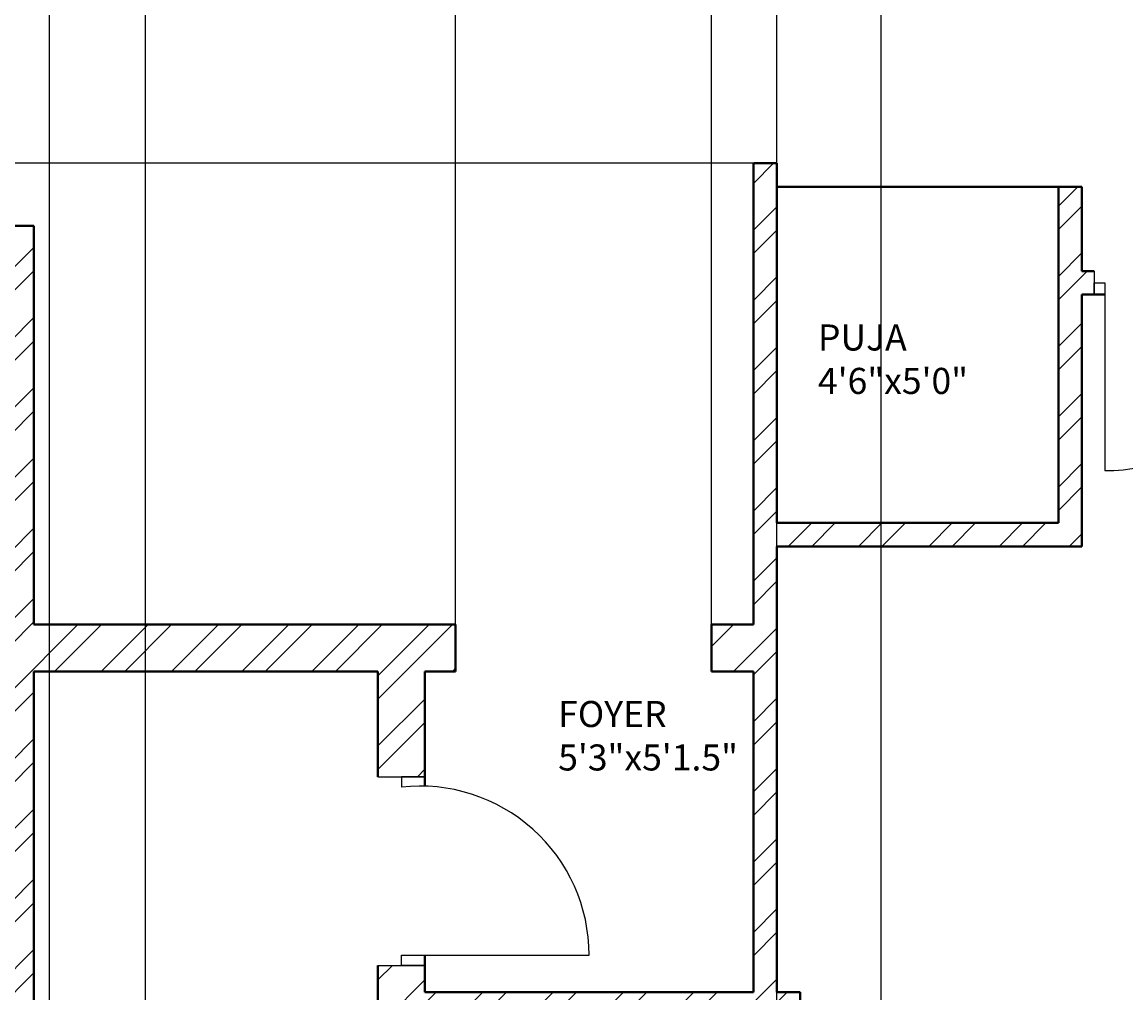
# Model space of a CAD drawing. Units: inches. Extents: x 1601 to 2297, y 1496 to 2631.
# Tile 46 of 57: x 1891 to 2102, y 2141 to 2327. Entities that reach past the tile are written whole.
import ezdxf

# ---------------------------------------------------------------- set-up
doc = ezdxf.new("R2010")
doc.units = ezdxf.units.IN
for name, color, linetype, lineweight in [('A-ANNO-DIMS', 2, 'Continuous', 18), ('A-AREA-IDEN', 7, 'Continuous', 18), ('A-DOOR', 21, 'Continuous', 25), ('A-WALL', 7, 'Continuous', 40), ('A-WALL-PATT', 215, 'Continuous', 13)]:
    doc.layers.add(name, color=color, linetype=linetype, lineweight=lineweight)
doc.styles.get("Standard").update_dxf_attribs({"font": 'arial.ttf'})
doc.dimstyles.get("Standard").update_dxf_attribs({"dimtxt": 0.18, "dimasz": 0.18, "dimexe": 0.18, "dimexo": 0.0625, "dimgap": 0.09, "dimtad": 0, "dimtih": 1, "dimtoh": 1, "dimdec": 4, "dimzin": 0, "dimdsep": 46, "dimtxsty": 'Standard', "dimcen": 0.09, "dimadec": 0, "dimazin": 0, "dimtfac": 1, "dimtdec": 4, "dimtofl": 0, "dimtmove": 0, "dimatfit": 3, "dimfxl": 1, "dimtolj": 1, "dimtzin": 0, "dimarcsym": 0})

# ---------------------------------------------------------------- blocks, each defined once
blk = doc.blocks.new('*D40')
at = {"layer": 'A-ANNO-DIMS', "color": 0, "lineweight": -2, "transparency": 16777216}
for p, q in [((2035.54, 1986.39), (2035.54, 2581.06)), ((2035.72, 2580.88), (2045.08, 2580.88)), ((2055.37, 2580.88), (2046.01, 2580.88)), ((2055.55, 1986.39), (2055.55, 2581.06))]:
    blk.add_line(p, q, dxfattribs=at)
at = {"layer": 'A-ANNO-DIMS', "color": 0, "transparency": 16777216}
for points in [[(2035.72, 2580.91), (2035.72, 2580.85), (2035.54, 2580.88)], [(2055.37, 2580.91), (2055.37, 2580.85), (2055.55, 2580.88)]]:
    blk.add_solid(points, dxfattribs=at)
at = {"layer": 'Defpoints', "color": 0, "transparency": 16777216}
for p in [(2055.55, 2580.88), (2035.54, 1986.33), (2055.55, 1986.33)]:
    blk.add_point(p, dxfattribs=at)
at = {"layer": 'A-ANNO-DIMS', "color": 0, "transparency": 16777216, "insert": (2045.54, 2580.88), "char_height": 0.18, "attachment_point": 5}
blk.add_mtext('\\A1;20.014', dxfattribs=at)
blk = doc.blocks.new('*D47')
at = {"layer": 'A-ANNO-DIMS', "color": 0, "lineweight": -2, "transparency": 16777216}
for p, q in [((1973.94, 2211.39), (1973.94, 2581.06)), ((1974.12, 2580.88), (1998.07, 2580.88)), ((2022.83, 2580.88), (1998.87, 2580.88)), ((2023.01, 2211.39), (2023.01, 2581.06))]:
    blk.add_line(p, q, dxfattribs=at)
at = {"layer": 'A-ANNO-DIMS', "color": 0, "transparency": 16777216}
for points in [[(1974.12, 2580.91), (1974.12, 2580.85), (1973.94, 2580.88)], [(2022.83, 2580.91), (2022.83, 2580.85), (2023.01, 2580.88)]]:
    blk.add_solid(points, dxfattribs=at)
at = {"layer": 'Defpoints', "color": 0, "transparency": 16777216}
for p in [(2023.01, 2580.88), (1973.94, 2211.33), (2023.01, 2211.33)]:
    blk.add_point(p, dxfattribs=at)
at = {"layer": 'A-ANNO-DIMS', "color": 0, "transparency": 16777216, "insert": (1998.47, 2580.88), "char_height": 0.18, "attachment_point": 5}
blk.add_mtext('\\A1;49.07', dxfattribs=at)
blk = doc.blocks.new('*D48')
at = {"layer": 'A-ANNO-DIMS', "color": 0, "lineweight": -2, "transparency": 16777216}
for p, q in [((2030.97, 2373.19), (1637.31, 2373.19)), ((1637.49, 2373.01), (1637.49, 2336.69)), ((1637.49, 2300.01), (1637.49, 2336.33)), ((2030.97, 2299.83), (1637.31, 2299.83))]:
    blk.add_line(p, q, dxfattribs=at)
at = {"layer": 'A-ANNO-DIMS', "color": 0, "transparency": 16777216}
for points in [[(1637.46, 2373.01), (1637.52, 2373.01), (1637.49, 2373.19)], [(1637.46, 2300.01), (1637.52, 2300.01), (1637.49, 2299.83)]]:
    blk.add_solid(points, dxfattribs=at)
at = {"layer": 'Defpoints', "color": 0, "transparency": 16777216}
for p in [(1637.49, 2373.19), (2031.04, 2373.19), (2031.04, 2299.83)]:
    blk.add_point(p, dxfattribs=at)
at = {"layer": 'A-ANNO-DIMS', "color": 0, "transparency": 16777216, "insert": (1637.49, 2336.51), "char_height": 0.18, "attachment_point": 5}
blk.add_mtext('\\A1;73.37', dxfattribs=at)
blk = doc.blocks.new('*D50')
at = {"layer": 'A-ANNO-DIMS', "color": 0, "lineweight": -2, "transparency": 16777216}
for p, q in [((1895.99, 2374.33), (1895.99, 1513.75)), ((1914.39, 2374.33), (1914.39, 1513.75)), ((1896.17, 1513.93), (1904.87, 1513.93)), ((1914.21, 1513.93), (1905.5, 1513.93))]:
    blk.add_line(p, q, dxfattribs=at)
at = {"layer": 'A-ANNO-DIMS', "color": 0, "transparency": 16777216}
for points in [[(1896.17, 1513.96), (1896.17, 1513.9), (1895.99, 1513.93)], [(1914.21, 1513.96), (1914.21, 1513.9), (1914.39, 1513.93)]]:
    blk.add_solid(points, dxfattribs=at)
at = {"layer": 'Defpoints', "color": 0, "transparency": 16777216}
for p in [(1895.99, 2374.4), (1914.39, 2374.4), (1914.39, 1513.93)]:
    blk.add_point(p, dxfattribs=at)
at = {"layer": 'A-ANNO-DIMS', "color": 0, "transparency": 16777216, "insert": (1905.19, 1513.93), "char_height": 0.18, "attachment_point": 5}
blk.add_mtext('\\A1;18.4', dxfattribs=at)

msp = doc.modelspace()

# ---------------------------------------------------------------- hatches: boundary and pattern name
at = {"layer": 'A-WALL-PATT'}
h = msp.add_hatch(dxfattribs=at)
h.set_pattern_fill('ANSI32', color=256)
h.paths.add_polyline_path([(1842.0336, 2528.0767), (1842.0336, 2532.3254), (1686.0373, 2532.3254), (1686.0373, 2492.9493), (1695.0373, 2492.9493), (1695.0373, 2523.3254), (1827.0373, 2523.3254), (1827.0373, 2416.8254), (1834.6225, 2416.8254), (1834.6225, 2419.0754), (1834.6225, 2421.3254), (1831.5373, 2421.3254), (1831.5373, 2523.3254), (1842.0336, 2523.3254)])
h.paths.add_polyline_path([(1695.0373, 2432.9493), (1686.0373, 2432.9493), (1686.0373, 2325.989), (1695.0373, 2325.989), (1695.0373, 2347.8254), (1827.0373, 2347.8254), (1827.0373, 2287.8254), (1823.2991, 2287.8254), (1823.2991, 2283.3254), (1847.9422, 2283.3254), (1847.9422, 2285.5754), (1847.9422, 2287.8254), (1831.5373, 2287.8254), (1831.5373, 2347.8254), (1846.9946, 2347.8254), (1846.9946, 2350.0754), (1846.9946, 2352.3254), (1695.0373, 2352.3254)])
h.paths.add_polyline_path([(1807.1169, 1573.5395), (2055.0405, 1573.5395), (2055.0405, 1610.6322), (1807.1169, 1610.6322)], flags=9)
h.paths.add_polyline_path([(1841.1631, 1712.7967), (1870.3957, 1712.7967), (1870.3957, 1731.454), (1841.1631, 1731.454)], flags=9)
h.paths.add_polyline_path([(2144.3862, 1772.185), (2191.0233, 1772.185), (2191.0233, 1790.8423), (2144.3862, 1790.8423)], flags=9)
h.paths.add_polyline_path([(2143.0128, 1827.3312), (2177.9958, 1827.3312), (2177.9958, 1845.9886), (2143.0128, 1845.9886)], flags=9)
h.paths.add_polyline_path([(2041.2439, 1833.5691), (2070.8516, 1833.5691), (2070.8516, 1852.2264), (2041.2439, 1852.2264)], flags=9)
h.paths.add_polyline_path([(2097.2791, 1947.0598), (2134.2061, 1947.0598), (2134.2061, 1965.7171), (2097.2791, 1965.7171)], flags=9)
h.paths.add_polyline_path([(2214.995, 1904.3124), (2214.995, 1942.2899), (2196.3376, 1942.2899), (2196.3376, 1904.3124)], flags=9)
h.paths.add_polyline_path([(2186.6284, 2043.8031), (2219.7935, 2043.8031), (2219.7935, 2062.4605), (2186.6284, 2062.4605)], flags=9)
h.paths.add_polyline_path([(2064.0877, 2031.616), (2097.4949, 2031.616), (2097.4949, 2050.2734), (2064.0877, 2050.2734)], flags=9)
h.paths.add_polyline_path([(1973.1349, 1986.0688), (2008.4009, 1986.0688), (2008.4009, 2004.7261), (1973.1349, 2004.7261)], flags=9)
h.paths.add_polyline_path([(1976.3676, 2106.9635), (2005.7469, 2106.9635), (2005.7469, 2125.6209), (1976.3676, 2125.6209)], flags=9)
h.paths.add_polyline_path([(1991.7852, 2180.4863), (2027.0513, 2180.4863), (2027.0513, 2199.1437), (1991.7852, 2199.1437)], flags=9)
h.paths.add_polyline_path([(2106.1801, 2187.9359), (2152.2101, 2187.9359), (2152.2101, 2206.5932), (2106.1801, 2206.5932)], flags=9)
h.paths.add_polyline_path([(2148.6686, 2262.2542), (2182.318, 2262.2542), (2182.318, 2280.9115), (2148.6686, 2280.9115)], flags=9)
h.paths.add_polyline_path([(2041.6327, 2252.8147), (2071.2405, 2252.8147), (2071.2405, 2271.4721), (2041.6327, 2271.4721)], flags=9)
h.paths.add_polyline_path([(2063.9734, 2375.4265), (2100.9004, 2375.4265), (2100.9004, 2394.0839), (2063.9734, 2394.0839)], flags=9)
h.paths.add_polyline_path([(2216.4955, 2330.9748), (2216.4955, 2370.2654), (2197.8381, 2370.2654), (2197.8381, 2330.9748)], flags=9)
h.paths.add_polyline_path([(2179.1416, 2485.8687), (2212.3067, 2485.8687), (2212.3067, 2504.5261), (2179.1416, 2504.5261)], flags=9)
h.paths.add_polyline_path([(2078.7442, 2471.1516), (2112.1514, 2471.1516), (2112.1514, 2489.809), (2078.7442, 2489.809)], flags=9)
h.paths.add_polyline_path([(1915.9631, 2329.4668), (1952.8902, 2329.4668), (1952.8902, 2348.1241), (1915.9631, 2348.1241)], flags=9)
h.paths.add_polyline_path([(1904.3189, 2499.6709), (1940.4512, 2499.6709), (1940.4512, 2518.3282), (1904.3189, 2518.3282)], flags=9)
h.paths.add_polyline_path([(1892.3665, 2100.4595), (1925.6374, 2100.4595), (1925.6374, 2119.1169), (1892.3665, 2119.1169)], flags=9)
h.paths.add_polyline_path([(1909.2984, 1805.9631), (1946.2254, 1805.9631), (1946.2254, 1824.6205), (1909.2984, 1824.6205)], flags=9)
h.paths.add_polyline_path([(1934.6056, 1658.616), (1970.738, 1658.616), (1970.738, 1677.2733), (1934.6056, 1677.2733)], flags=9)
h.paths.add_polyline_path([(1711.2052, 1789.8902), (1750.0456, 1789.8902), (1750.0456, 1808.5476), (1711.2052, 1808.5476)], flags=9)
h.paths.add_polyline_path([(1742.7874, 1854.6743), (1771.9449, 1854.6743), (1771.9449, 1873.3317), (1742.7874, 1873.3317)], flags=9)
h.paths.add_polyline_path([(1807.3592, 1997.7912), (1850.1116, 1997.7912), (1850.1116, 2016.4486), (1807.3592, 2016.4486)], flags=9)
h.paths.add_polyline_path([(1717.4579, 2237.7844), (1760.2103, 2237.7844), (1760.2103, 2256.4417), (1717.4579, 2256.4417)], flags=9)
h.paths.add_polyline_path([(1780.9285, 2324.0623), (1810.086, 2324.0623), (1810.086, 2342.7197), (1780.9285, 2342.7197)], flags=25)
h.paths.add_polyline_path([(1837.696, 2449.2024), (1866.9286, 2449.2024), (1866.9286, 2467.8598), (1837.696, 2467.8598)], flags=9)
h.paths.add_polyline_path([(1712.7752, 2484.9404), (1751.6156, 2484.9404), (1751.6156, 2503.5977), (1712.7752, 2503.5977)], flags=25)
h = msp.add_hatch(dxfattribs=at)
h.set_pattern_fill('ANSI32', color=256)
h.paths.add_polyline_path([(1973.9371, 2211.3254), (1893.0373, 2211.3254), (1893.0373, 2287.8254), (1884.6167, 2287.8254), (1884.6167, 2285.5754), (1884.6167, 2283.3254), (1888.5373, 2283.3254), (1888.5373, 2145.3254), (1695.0373, 2145.3254), (1695.0373, 2173.8724), (1690.5373, 2173.8724), (1686.0373, 2173.8724), (1686.0373, 2136.3254), (1722.5687, 2136.3254), (1722.5687, 2117.4352), (1731.5687, 2117.4352), (1731.5687, 2136.3254), (1893.0373, 2136.3254), (1893.0373, 2202.3254), (1959.0373, 2202.3254), (1959.0373, 2182.1303), (1968.0373, 2182.1303), (1968.0373, 2202.3254), (1973.9371, 2202.3254)])
h.paths.add_polyline_path([(2094.0373, 2274.6364), (2096.4294, 2274.6364), (2096.4294, 2276.8864), (2096.4294, 2279.1364), (2094.0373, 2279.1364), (2094.0373, 2290.8254), (2094.0373, 2295.3254), (2089.5373, 2295.3254), (2089.5373, 2230.8254), (2035.5373, 2230.8254), (2035.5373, 2299.8254), (2031.0373, 2299.8254), (2031.0373, 2211.3254), (2023.0065, 2211.3254), (2023.0065, 2202.3254), (2031.0373, 2202.3254), (2031.0373, 2140.8254), (1968.0373, 2140.8254), (1968.0373, 2145.9106), (1963.5373, 2145.9106), (1959.0373, 2145.9106), (1959.0373, 2116.839), (1963.5373, 2116.839), (1968.0373, 2116.839), (1968.0373, 2131.8254), (2031.0373, 2131.8254), (2031.0373, 2094.3254), (2031.0373, 2085.3254), (2031.0373, 2056.8254), (1968.0373, 2056.8254), (1968.0373, 2070.4947), (1963.5373, 2070.4947), (1959.0373, 2070.4947), (1959.0373, 2040.3029), (1968.0373, 2040.3029), (1968.0373, 2047.8254), (2031.0373, 2047.8254), (2031.0373, 1983.3254), (2031.0373, 1978.8254), (2021.1979, 1978.8254), (2021.1979, 1974.3254), (2031.0373, 1974.3254), (2031.0373, 1954.3528), (2035.5373, 1954.3528), (2035.5373, 1974.3254), (2035.5373, 1981.8254), (2055.5513, 1981.8254), (2055.5513, 1986.3254), (2035.5373, 1986.3254), (2035.5373, 2047.8254), (2040.0373, 2047.8254), (2040.0373, 2085.3254), (2040.0373, 2094.3254), (2040.0373, 2140.8254), (2035.5373, 2140.8254), (2035.5373, 2226.3254), (2089.5373, 2226.3254), (2094.0373, 2226.3254)])
h.paths.add_polyline_path([(2226.0373, 2230.8254), (2134.5373, 2230.8254), (2134.5373, 2233.5437), (2130.0373, 2233.5437), (2130.0373, 2226.3254), (2134.5373, 2226.3254), (2226.0373, 2226.3254)])
h.paths.add_polyline_path([(1807.1169, 1573.5395), (2055.0405, 1573.5395), (2055.0405, 1610.6322), (1807.1169, 1610.6322)], flags=9)
h.paths.add_polyline_path([(1841.1631, 1712.7967), (1870.3957, 1712.7967), (1870.3957, 1731.454), (1841.1631, 1731.454)], flags=9)
h.paths.add_polyline_path([(2144.3862, 1772.185), (2191.0233, 1772.185), (2191.0233, 1790.8423), (2144.3862, 1790.8423)], flags=9)
h.paths.add_polyline_path([(2143.0128, 1827.3312), (2177.9958, 1827.3312), (2177.9958, 1845.9886), (2143.0128, 1845.9886)], flags=9)
h.paths.add_polyline_path([(2041.2439, 1833.5691), (2070.8516, 1833.5691), (2070.8516, 1852.2264), (2041.2439, 1852.2264)], flags=9)
h.paths.add_polyline_path([(2097.2791, 1947.0598), (2134.2061, 1947.0598), (2134.2061, 1965.7171), (2097.2791, 1965.7171)], flags=9)
h.paths.add_polyline_path([(2214.995, 1904.3124), (2214.995, 1942.2899), (2196.3376, 1942.2899), (2196.3376, 1904.3124)], flags=9)
h.paths.add_polyline_path([(2186.6284, 2043.8031), (2219.7935, 2043.8031), (2219.7935, 2062.4605), (2186.6284, 2062.4605)], flags=9)
h.paths.add_polyline_path([(2064.0877, 2031.616), (2097.4949, 2031.616), (2097.4949, 2050.2734), (2064.0877, 2050.2734)], flags=9)
h.paths.add_polyline_path([(1973.1349, 1986.0688), (2008.4009, 1986.0688), (2008.4009, 2004.7261), (1973.1349, 2004.7261)], flags=25)
h.paths.add_polyline_path([(1976.3676, 2106.9635), (2005.7469, 2106.9635), (2005.7469, 2125.6209), (1976.3676, 2125.6209)], flags=25)
h.paths.add_polyline_path([(1991.7852, 2180.4863), (2027.0513, 2180.4863), (2027.0513, 2199.1437), (1991.7852, 2199.1437)], flags=25)
h.paths.add_polyline_path([(2106.1801, 2187.9359), (2152.2101, 2187.9359), (2152.2101, 2206.5932), (2106.1801, 2206.5932)], flags=9)
h.paths.add_polyline_path([(2148.6686, 2262.2542), (2182.318, 2262.2542), (2182.318, 2280.9115), (2148.6686, 2280.9115)], flags=9)
h.paths.add_polyline_path([(2041.6327, 2252.8147), (2071.2405, 2252.8147), (2071.2405, 2271.4721), (2041.6327, 2271.4721)], flags=25)
h.paths.add_polyline_path([(2063.9734, 2375.4265), (2100.9004, 2375.4265), (2100.9004, 2394.0839), (2063.9734, 2394.0839)], flags=9)
h.paths.add_polyline_path([(2216.4955, 2330.9748), (2216.4955, 2370.2654), (2197.8381, 2370.2654), (2197.8381, 2330.9748)], flags=9)
h.paths.add_polyline_path([(2179.1416, 2485.8687), (2212.3067, 2485.8687), (2212.3067, 2504.5261), (2179.1416, 2504.5261)], flags=9)
h.paths.add_polyline_path([(2078.7442, 2471.1516), (2112.1514, 2471.1516), (2112.1514, 2489.809), (2078.7442, 2489.809)], flags=9)
h.paths.add_polyline_path([(1915.9631, 2329.4668), (1952.8902, 2329.4668), (1952.8902, 2348.1241), (1915.9631, 2348.1241)], flags=9)
h.paths.add_polyline_path([(1904.3189, 2499.6709), (1940.4512, 2499.6709), (1940.4512, 2518.3282), (1904.3189, 2518.3282)], flags=9)
h.paths.add_polyline_path([(1892.3665, 2100.4595), (1925.6374, 2100.4595), (1925.6374, 2119.1169), (1892.3665, 2119.1169)], flags=9)
h.paths.add_polyline_path([(1909.2984, 1805.9631), (1946.2254, 1805.9631), (1946.2254, 1824.6205), (1909.2984, 1824.6205)], flags=9)
h.paths.add_polyline_path([(1934.6056, 1658.616), (1970.738, 1658.616), (1970.738, 1677.2733), (1934.6056, 1677.2733)], flags=9)
h.paths.add_polyline_path([(1711.2052, 1789.8902), (1750.0456, 1789.8902), (1750.0456, 1808.5476), (1711.2052, 1808.5476)], flags=9)
h.paths.add_polyline_path([(1742.7874, 1854.6743), (1771.9449, 1854.6743), (1771.9449, 1873.3317), (1742.7874, 1873.3317)], flags=9)
h.paths.add_polyline_path([(1807.3592, 1997.7912), (1850.1116, 1997.7912), (1850.1116, 2016.4486), (1807.3592, 2016.4486)], flags=9)
h.paths.add_polyline_path([(1717.4579, 2237.7844), (1760.2103, 2237.7844), (1760.2103, 2256.4417), (1717.4579, 2256.4417)], flags=25)
h.paths.add_polyline_path([(1780.9285, 2324.0623), (1810.086, 2324.0623), (1810.086, 2342.7197), (1780.9285, 2342.7197)], flags=9)
h.paths.add_polyline_path([(1837.696, 2449.2024), (1866.9286, 2449.2024), (1866.9286, 2467.8598), (1837.696, 2467.8598)], flags=9)
h.paths.add_polyline_path([(1712.7752, 2484.9404), (1751.6156, 2484.9404), (1751.6156, 2503.5977), (1712.7752, 2503.5977)], flags=9)
h = msp.add_hatch(dxfattribs=at)
h.set_pattern_fill('ANSI32', color=256)
h.paths.add_polyline_path([(2230.5373, 1861.8254), (2182.5373, 1861.8254), (2182.5373, 1885.3637), (2178.0373, 1885.3637), (2178.0373, 1861.8254), (2166.0373, 1861.8254), (2134.5373, 1861.8254), (2130.0373, 1861.8254), (2130.0373, 1841.4682), (2126.8833, 1841.4682), (2126.8833, 1836.9682), (2130.0373, 1836.9682), (2130.0373, 1822.7302), (2134.5373, 1822.7302), (2134.5373, 1857.3254), (2166.0373, 1857.3254), (2226.0373, 1857.3254), (2226.0373, 1846.1155), (2230.5373, 1846.1155)])
h.paths.add_polyline_path([(2226.0373, 1797.3254), (2134.5373, 1797.3254), (2134.5373, 1800.6636), (2132.2873, 1800.6636), (2130.0373, 1800.6636), (2130.0373, 1797.3254), (2130.0373, 1792.8254), (2167.7264, 1792.8254), (2226.0373, 1792.8254)])
h.paths.add_polyline_path([(2230.5373, 1822.1155), (2226.0373, 1822.1155), (2226.0373, 1760.8563), (2230.5373, 1760.8563)])
h.paths.add_polyline_path([(2230.5373, 1700.8563), (2226.0373, 1700.8563), (2226.0373, 1644.3254), (2140.2517, 1644.3254), (2140.2517, 1635.3254), (2230.5373, 1635.3254)])
h.paths.add_polyline_path([(2080.2517, 1639.8254), (2080.2517, 1644.3254), (2035.5373, 1644.3254), (2035.5373, 1792.8254), (2094.0373, 1792.8254), (2094.0373, 1797.3254), (2094.0373, 1836.9682), (2097.1057, 1836.9682), (2097.1057, 1839.2182), (2097.1057, 1841.4682), (2094.0373, 1841.4682), (2094.0373, 1862.2276), (2089.5373, 1862.2276), (2089.5373, 1797.3254), (2035.5373, 1797.3254), (2035.5373, 1857.3254), (2035.5373, 1885.0916), (2031.0373, 1885.0916), (2031.0373, 1710.3254), (2012.329, 1710.3254), (2012.329, 1701.3254), (2031.0373, 1701.3254), (2031.0373, 1644.3254), (2031.0373, 1635.3254), (2080.2517, 1635.3254)])
h.paths.add_polyline_path([(1836.0373, 1653.2033), (1842.6171, 1653.2033), (1842.6171, 1657.7033), (1842.6171, 1662.2033), (1831.5373, 1662.2033), (1831.5373, 1764.2033), (1835.3881, 1764.2033), (1835.3881, 1766.4533), (1835.3881, 1768.7033), (1831.5373, 1768.7033), (1827.0373, 1768.7033), (1827.0373, 1662.2033), (1827.0373, 1635.3254), (1836.0373, 1635.3254)])
h.paths.add_polyline_path([(1893.0373, 1701.3254), (1907.193, 1701.3254), (1907.193, 1705.8254), (1907.193, 1710.3254), (1893.0373, 1710.3254), (1893.0373, 1819.8254), (1882.6444, 1819.8254), (1882.6444, 1817.5754), (1882.6444, 1815.3254), (1888.5373, 1815.3254), (1888.5373, 1662.2033), (1884.0373, 1662.2033), (1866.6171, 1662.2033), (1866.6171, 1653.2033), (1882.391, 1653.2033), (1884.0373, 1653.2033), (1884.0373, 1635.3254), (1893.0373, 1635.3254)])
h.paths.add_polyline_path([(1739.3335, 1639.8254), (1739.3335, 1644.3254), (1695.0373, 1644.3254), (1695.0373, 1702.0135), (1690.5373, 1702.0135), (1686.0373, 1702.0135), (1686.0373, 1635.3254), (1739.3335, 1635.3254)])
h.paths.add_polyline_path([(1827.0373, 1644.3254), (1799.3335, 1644.3254), (1799.3335, 1635.3254), (1827.0373, 1635.3254)])
h.paths.add_polyline_path([(1695.0373, 1815.3254), (1849.2759, 1815.3254), (1849.2759, 1819.8254), (1807.5373, 1819.8254), (1807.5373, 1879.8254), (1851.1533, 1879.8254), (1851.1533, 1882.0754), (1851.1533, 1884.3254), (1799.3405, 1884.3254), (1799.3405, 1882.0754), (1799.3405, 1879.8254), (1803.0373, 1879.8254), (1803.0373, 1819.8254), (1695.0373, 1819.8254), (1695.0373, 1835.0458), (1690.5373, 1835.0458), (1686.0373, 1835.0458), (1686.0373, 1766.1753), (1695.0373, 1766.1753)])
h.paths.add_polyline_path([(1775.8157, 1884.3254), (1695.0373, 1884.3254), (1695.0373, 1912.9526), (1690.5373, 1912.9526), (1686.0373, 1912.9526), (1686.0373, 1859.0458), (1695.0373, 1859.0458), (1695.0373, 1879.8254), (1775.8157, 1879.8254)])
h.paths.add_polyline_path([(1893.0373, 2031.3254), (1731.5687, 2031.3254), (1731.5687, 2057.4352), (1722.5687, 2057.4352), (1722.5687, 2031.3254), (1686.0373, 2031.3254), (1686.0373, 1972.9526), (1695.0373, 1972.9526), (1695.0373, 2022.3254), (1888.5373, 2022.3254), (1888.5373, 1884.3254), (1883.4996, 1884.3254), (1883.4996, 1879.8254), (1893.0373, 1879.8254), (1893.0373, 1974.3254), (1976.6199, 1974.3254), (1976.6199, 1978.8254), (1968.0373, 1978.8254), (1968.0373, 1983.3254), (1968.0373, 2008.4756), (1963.5373, 2008.4756), (1959.0373, 2008.4756), (1959.0373, 1983.3254), (1893.0373, 1983.3254)])
h.paths.add_polyline_path([(2230.5373, 2140.4745), (2226.0373, 2140.4745), (2226.0373, 2094.3254), (2040.0373, 2094.3254), (2040.0373, 2085.3254), (2178.0373, 2085.3254), (2178.0373, 2065.6965), (2182.5373, 2065.6965), (2182.5373, 2085.3254), (2226.0373, 2085.3254), (2226.0373, 1986.3254), (2211.2679, 1986.3254), (2211.2679, 1981.8254), (2230.5373, 1981.8254)])
h.paths.add_polyline_path([(2187.6292, 1986.3254), (2182.5373, 1986.3254), (2182.5373, 2029.6965), (2178.0373, 2029.6965), (2178.0373, 1986.3254), (2099.05, 1986.3254), (2099.05, 1981.8254), (2178.0373, 1981.8254), (2178.0373, 1969.3637), (2182.5373, 1969.3637), (2182.5373, 1981.8254), (2187.6292, 1981.8254), (2187.6292, 1984.0754)])
h.paths.add_polyline_path([(1807.1169, 1573.5395), (2055.0405, 1573.5395), (2055.0405, 1610.6322), (1807.1169, 1610.6322)], flags=9)
h.paths.add_polyline_path([(1841.1631, 1712.7967), (1870.3957, 1712.7967), (1870.3957, 1731.454), (1841.1631, 1731.454)], flags=9)
h.paths.add_polyline_path([(2144.3862, 1772.185), (2191.0233, 1772.185), (2191.0233, 1790.8423), (2144.3862, 1790.8423)], flags=9)
h.paths.add_polyline_path([(2143.0128, 1827.3312), (2177.9958, 1827.3312), (2177.9958, 1845.9886), (2143.0128, 1845.9886)], flags=25)
h.paths.add_polyline_path([(2041.2439, 1833.5691), (2070.8516, 1833.5691), (2070.8516, 1852.2264), (2041.2439, 1852.2264)], flags=25)
h.paths.add_polyline_path([(2097.2791, 1947.0598), (2134.2061, 1947.0598), (2134.2061, 1965.7171), (2097.2791, 1965.7171)], flags=9)
h.paths.add_polyline_path([(2214.995, 1904.3124), (2214.995, 1942.2899), (2196.3376, 1942.2899), (2196.3376, 1904.3124)], flags=9)
h.paths.add_polyline_path([(2186.6284, 2043.8031), (2219.7935, 2043.8031), (2219.7935, 2062.4605), (2186.6284, 2062.4605)], flags=25)
h.paths.add_polyline_path([(2064.0877, 2031.616), (2097.4949, 2031.616), (2097.4949, 2050.2734), (2064.0877, 2050.2734)], flags=25)
h.paths.add_polyline_path([(1973.1349, 1986.0688), (2008.4009, 1986.0688), (2008.4009, 2004.7261), (1973.1349, 2004.7261)], flags=9)
h.paths.add_polyline_path([(1976.3676, 2106.9635), (2005.7469, 2106.9635), (2005.7469, 2125.6209), (1976.3676, 2125.6209)], flags=9)
h.paths.add_polyline_path([(1991.7852, 2180.4863), (2027.0513, 2180.4863), (2027.0513, 2199.1437), (1991.7852, 2199.1437)], flags=9)
h.paths.add_polyline_path([(2106.1801, 2187.9359), (2152.2101, 2187.9359), (2152.2101, 2206.5932), (2106.1801, 2206.5932)], flags=9)
h.paths.add_polyline_path([(2148.6686, 2262.2542), (2182.318, 2262.2542), (2182.318, 2280.9115), (2148.6686, 2280.9115)], flags=9)
h.paths.add_polyline_path([(2041.6327, 2252.8147), (2071.2405, 2252.8147), (2071.2405, 2271.4721), (2041.6327, 2271.4721)], flags=9)
h.paths.add_polyline_path([(2063.9734, 2375.4265), (2100.9004, 2375.4265), (2100.9004, 2394.0839), (2063.9734, 2394.0839)], flags=9)
h.paths.add_polyline_path([(2216.4955, 2330.9748), (2216.4955, 2370.2654), (2197.8381, 2370.2654), (2197.8381, 2330.9748)], flags=9)
h.paths.add_polyline_path([(2179.1416, 2485.8687), (2212.3067, 2485.8687), (2212.3067, 2504.5261), (2179.1416, 2504.5261)], flags=9)
h.paths.add_polyline_path([(2078.7442, 2471.1516), (2112.1514, 2471.1516), (2112.1514, 2489.809), (2078.7442, 2489.809)], flags=9)
h.paths.add_polyline_path([(1915.9631, 2329.4668), (1952.8902, 2329.4668), (1952.8902, 2348.1241), (1915.9631, 2348.1241)], flags=9)
h.paths.add_polyline_path([(1904.3189, 2499.6709), (1940.4512, 2499.6709), (1940.4512, 2518.3282), (1904.3189, 2518.3282)], flags=9)
h.paths.add_polyline_path([(1892.3665, 2100.4595), (1925.6374, 2100.4595), (1925.6374, 2119.1169), (1892.3665, 2119.1169)], flags=9)
h.paths.add_polyline_path([(1909.2984, 1805.9631), (1946.2254, 1805.9631), (1946.2254, 1824.6205), (1909.2984, 1824.6205)], flags=9)
h.paths.add_polyline_path([(1934.6056, 1658.616), (1970.738, 1658.616), (1970.738, 1677.2733), (1934.6056, 1677.2733)], flags=9)
h.paths.add_polyline_path([(1711.2052, 1789.8902), (1750.0456, 1789.8902), (1750.0456, 1808.5476), (1711.2052, 1808.5476)], flags=25)
h.paths.add_polyline_path([(1742.7874, 1854.6743), (1771.9449, 1854.6743), (1771.9449, 1873.3317), (1742.7874, 1873.3317)], flags=25)
h.paths.add_polyline_path([(1807.3592, 1997.7912), (1850.1116, 1997.7912), (1850.1116, 2016.4486), (1807.3592, 2016.4486)], flags=25)
h.paths.add_polyline_path([(1717.4579, 2237.7844), (1760.2103, 2237.7844), (1760.2103, 2256.4417), (1717.4579, 2256.4417)], flags=9)
h.paths.add_polyline_path([(1780.9285, 2324.0623), (1810.086, 2324.0623), (1810.086, 2342.7197), (1780.9285, 2342.7197)], flags=9)
h.paths.add_polyline_path([(1837.696, 2449.2024), (1866.9286, 2449.2024), (1866.9286, 2467.8598), (1837.696, 2467.8598)], flags=9)
h.paths.add_polyline_path([(1712.7752, 2484.9404), (1751.6156, 2484.9404), (1751.6156, 2503.5977), (1712.7752, 2503.5977)], flags=9)

# ---------------------------------------------------------------- linework, layer by layer
at = {"layer": 'A-DOOR'}
for p, q in [((2096.4294, 2279.1364), (2096.4294, 2274.6364)), ((2096.4294, 2274.6364), (2096.4294, 2276.8864)), ((2096.4294, 2276.8864), (2098.4294, 2276.8864)), ((2098.4294, 2276.8864), (2098.4294, 2240.8864)), ((1959.0373, 2182.1303), (1968.0373, 2182.1303)), ((1968.0373, 2182.1303), (1963.5373, 2182.1303)), ((1963.5373, 2182.1303), (1963.5373, 2180.1303)), ((1963.5373, 2145.9106), (1963.5373, 2147.9106)), ((1963.5373, 2147.9106), (1999.5373, 2147.9106)), ((1959.0373, 2145.9106), (1968.0373, 2145.9106)), ((1968.0373, 2145.9106), (1963.5373, 2145.9106))]:
    msp.add_line(p, q, dxfattribs=at)
for centre, radius, start, end in [((2098.9928, 2269.8227), 28.9418, 268.884453, 18.772337), ((1967.1191, 2147.9106), 32.4182, 0, 96.34347)]:
    msp.add_arc(centre, radius, start, end, dxfattribs=at)
at = {"layer": 'A-WALL'}
for p, q in [((2035.5373, 2299.8254), (2031.0373, 2299.8254)), ((2031.0373, 2299.8254), (2031.0373, 2211.3254)), ((2035.5373, 2230.8254), (2035.5373, 2299.8254)), ((2094.0373, 2295.3254), (2035.5373, 2295.3254)), ((2089.5373, 2295.3254), (2089.5373, 2230.8254)), ((2094.0373, 2290.8254), (2094.0373, 2295.3254)), ((2094.0373, 2279.1364), (2094.0373, 2290.8254)), ((1884.6167, 2287.8254), (1893.0373, 2287.8254)), ((1893.0373, 2287.8254), (1893.0373, 2211.3254)), ((2094.0373, 2279.1364), (2096.4294, 2279.1364)), ((2094.0373, 2226.3254), (2094.0373, 2274.6364)), ((2098.4294, 2274.6364), (2094.0373, 2274.6364)), ((2035.5373, 2239.8254), (2035.5373, 2235.3254)), ((2089.5373, 2230.8254), (2035.5373, 2230.8254)), ((2035.5373, 2140.8254), (2035.5373, 2226.3254)), ((2035.5373, 2226.3254), (2089.5373, 2226.3254)), ((2089.5373, 2226.3254), (2094.0373, 2226.3254)), ((1893.0373, 2211.3254), (1973.9371, 2211.3254)), ((1973.9371, 2202.3254), (1973.9371, 2211.3254)), ((2023.0065, 2211.3254), (2023.0065, 2202.3254)), ((2023.0065, 2211.3254), (2031.0373, 2211.3254)), ((1893.0373, 2202.3254), (1959.0373, 2202.3254)), ((1893.0373, 2202.3254), (1893.0373, 2136.3254)), ((1959.0373, 2202.3254), (1959.0373, 2182.1303)), ((1968.0373, 2202.3254), (1973.9371, 2202.3254)), ((1968.0373, 2180.3158), (1968.0373, 2202.3254)), ((2023.0065, 2202.3254), (2031.0373, 2202.3254)), ((2031.0373, 2202.3254), (2031.0373, 2140.8254)), ((1968.0373, 2140.8254), (1968.0373, 2147.9106)), ((1959.0373, 2145.9106), (1959.0373, 2116.839)), ((1968.0373, 2140.8254), (2031.0373, 2140.8254)), ((2035.5373, 2140.8254), (2040.0373, 2140.8254)), ((2040.0373, 2140.8254), (2040.0373, 2094.3254))]:
    msp.add_line(p, q, dxfattribs=at)

# ---------------------------------------------------------------- texts
at = {"layer": 'A-AREA-IDEN', "char_height": 5, "attachment_point": 1}
for s, width, insert in [('PUJA\\P4\'6"x5\'0"', 32.479778, (2043.4216, 2268.8988)), ('FOYER\\P5\'3"x5\'1.5"', 21.280395, (1993.6082, 2196.659))]:
    msp.add_mtext_dynamic_manual_height_columns(s, width=width, gutter_width=12.5, heights=[0], dxfattribs=dict(at, insert=insert))

# ---------------------------------------------------------------- dimensions: what is measured, and where the dimension line sits
at = {"layer": 'A-ANNO-DIMS'}
for base, p1, p2, override, picture, middle in [((2023.0065, 2580.8754), (1973.9371, 2211.3254), (2023.0065, 2211.3254), {"dimdec": 2, "dimlfac": 1, "dimrnd": 0, "dimzin": 0, "dimdsep": 46, "dimlunit": 2}, '*D47', (1998.4718, 2580.8754)), ((2055.5513, 2580.8754), (2035.5373, 1986.3254), (2055.5513, 1986.3254), {"dimdec": 3, "dimlfac": 1, "dimrnd": 0, "dimzin": 0, "dimdsep": 46, "dimlunit": 2}, '*D40', (2045.5443, 2580.8754)), ((1914.3895, 1513.9279), (1895.9902, 2374.3952), (1914.3895, 2374.3952), {"dimdec": 1, "dimlfac": 1, "dimrnd": 0, "dimzin": 0, "dimdsep": 46, "dimlunit": 2}, '*D50', (1905.1899, 1513.9279))]:
    dim = msp.add_linear_dim(base=base, p1=p1, p2=p2, dimstyle='Standard', override=override, dxfattribs=at)
    dim.commit()
    dim.dimension.update_dxf_attribs({"geometry": picture, "text_midpoint": middle})
dim = msp.add_linear_dim(base=(1637.4873, 2373.1914), p1=(2031.0373, 2299.8254), p2=(2031.0373, 2373.1914), angle=90, dimstyle='Standard', override={"dimdec": 2, "dimlfac": 1, "dimrnd": 0, "dimzin": 0, "dimdsep": 46, "dimlunit": 2}, dxfattribs=at)
dim.commit()
dim.dimension.update_dxf_attribs({"geometry": '*D48', "text_midpoint": (1637.4873, 2336.5084)})

doc.saveas('drawing.dxf')
